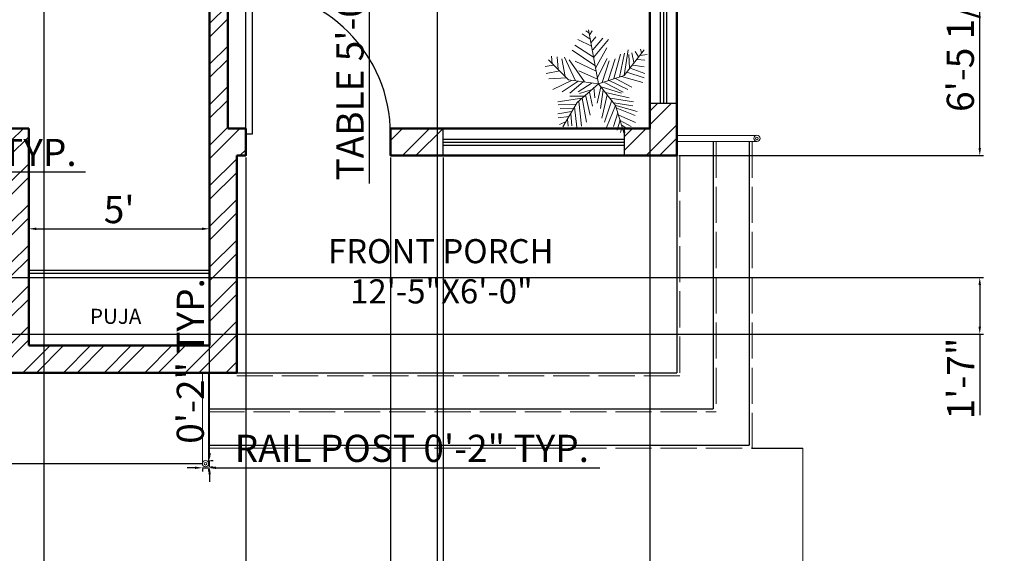
# Model space of a CAD drawing. Units: inches. Extents: x 635 to 1184, y 1837 to 2697.
# Tile 3 of 6: x 857 to 1184, y 2024 to 2201. Entities that reach past the tile are written whole.
import ezdxf

# ---------------------------------------------------------------- set-up
doc = ezdxf.new("R2010")
doc.units = ezdxf.units.IN
doc.linetypes.add('ACAD_ISO02W100', pattern=[15, 12, -3])
for name, color, linetype, lineweight in [('A-ANNO-DIMS', 2, 'Continuous', 18), ('A-ANNO-SYMB', 7, 'Continuous', 18), ('A-AREA-IDEN', 7, 'Continuous', 25), ('A-CSWK', 8, 'Continuous', 25), ('A-DOOR', 4, 'Continuous', 25), ('A-FLOR-RAIL', 7, 'Continuous', 18), ('A-FLOR-STRS', 7, 'Continuous', 25), ('A-FLOR-STRS-HIDN', 8, 'ACAD_ISO02W100', 13), ('A-GLAZ', 244, 'Continuous', 25), ('A-WALL', 7, 'Continuous', 50), ('A-WALL-PATT', 252, 'Continuous', 13), ('C-ROAD', 8, 'Continuous', 25), ('L-PLNT', 94, 'Continuous', 13)]:
    doc.layers.add(name, color=color, linetype=linetype, lineweight=lineweight)
doc.styles.get("Standard").update_dxf_attribs({"font": 'arial.ttf'})
doc.dimstyles.new('ISO-25', dxfattribs={"dimtxt": 9, "dimasz": 2.5, "dimexe": 1.25, "dimexo": 0.625, "dimtad": 1, "dimlunit": 3, "dimtxsty": 'Standard', "dimcen": 2.5, "dimadec": 0, "dimazin": 0, "dimtfac": 1, "dimtmove": 0, "dimatfit": 3, "dimfxl": 1, "dimarcsym": 0})

# ---------------------------------------------------------------- blocks, each defined once
blk = doc.blocks.new('*U3')
for p, q in [((0, 0), (0, -6)), ((40, 0), (40, -6))]:
    blk.add_line(p, q)
blk.add_lwpolyline([(0, 0), (0, 40), (1.75, 40), (1.75, 0)], close=True)
blk.add_arc((0, 0), 40, 0, 90)
blk = doc.blocks.new('*U15')
for p, q in [((-8.737, 47.138), (-17.069, 52.711)), ((-10.186, 53.64), (-13.084, 55.962)), ((0, 0), (-10.5, 57)), ((-9.099, 51.782), (-6.563, 55.962)), ((-7.288, 39.707), (-21.778, 46.673)), ((-7.65, 43.423), (-2.578, 49.46)), ((-5.839, 35.992), (4.667, 48.067)), ((-5.114, 27.632), (10.463, 46.673)), ((-3.665, 19.273), (-27.574, 35.527)), ((-5.114, 28.097), (-24.676, 40.636)), ((-2.941, 16.486), (8.652, 37.85)), ((16.259, 5.805), (23.142, 31.348)), ((22.055, 7.198), (27.489, 32.277)), ((27, 9), (48, 36)), ((27.127, 9.056), (31.112, 35.992)), ((35.096, 32.741), (37.27, 22.524)), ((38.719, 34.134), (41.979, 28.561)), ((44.153, 36.456), (45.239, 32.741)), ((-31.5, 4.5), (-52.5, 25.5)), ((-48.585, 21.131), (-49.309, 29.026)), ((-43.513, 28.561), (-42.427, 15.558)), ((-38.442, 26.239), (-34.819, 7.663)), ((-35.544, 28.097), (-24.314, 3.947)), ((-14.533, 2.09), (-30.834, 25.31)), ((-24.314, 23.917), (-2.941, 13.7)), ((-1.129, 6.734), (9.014, 26.704)), ((3.942, 1.625), (11.187, 24.381)), ((10.101, 3.483), (17.708, 26.239)), ((31.836, 30.883), (32.561, 16.486)), ((40.53, 25.775), (48.862, 24.846)), ((43.791, 29.954), (51.036, 30.883)), ((-47.498, 19.737), (-55.83, 18.344)), ((-40.615, 13.7), (-55.105, 10.913)), ((-20.691, 13.7), (-1.129, 4.876)), ((29.662, 12.307), (48.137, 6.269)), ((33.285, 16.486), (48.862, 10.913)), ((36.183, 19.737), (48.137, 17.88)), ((-33.37, 6.269), (-52.207, 5.34)), ((-28.299, 3.483), (-47.86, -5.805)), ((-21.416, 3.018), (-38.079, -8.128)), ((0, 0), (-31.5, 4.5)), ((-15.982, 2.09), (-30.11, -9.521)), ((0, 0), (-22.5, -19.5)), ((-6.563, 1.161), (-21.416, -8.128)), ((0, 0), (27, 9)), ((0, 0), (18, -22.5)), ((6.478, 1.625), (26.04, -8.592)), ((11.187, 3.483), (30.749, -5.805)), ((18.07, 5.805), (35.096, -3.483)), ((24.229, 7.663), (46.688, 1.625)), ((-6.563, -5.805), (-19.967, -9.985)), ((-9.461, -8.592), (-6.201, -23.453)), ((-4.752, -3.483), (-3.665, -14.629)), ((2.493, -3.019), (-1.491, -20.202)), ((1.769, -2.555), (24.229, -9.521)), ((5.029, -6.27), (2.131, -25.775)), ((7.565, -9.056), (32.198, -14.629)), ((-17.431, -15.094), (-42.789, -18.809)), ((-22.5, -19.5), (-37.5, -45)), ((-15.257, -12.772), (-30.11, -12.772)), ((-20.691, -18.345), (-17.793, -44.352)), ((-17.069, -15.094), (-12.721, -40.172)), ((-13.446, -11.378), (-8.737, -32.741)), ((9.014, -11.378), (3.58, -35.992)), ((14.085, -16.951), (6.478, -40.172)), ((12.274, -15.094), (36.907, -18.809)), ((16.259, -19.738), (36.183, -22.989)), ((-28.299, -29.026), (-42.789, -31.348)), ((-24.314, -21.596), (-42.427, -22.06)), ((-26.849, -26.24), (-40.253, -25.775)), ((-29.023, -30.884), (-27.936, -43.887)), ((-25.038, -23.918), (-22.865, -45.281)), ((18.07, -22.524), (8.289, -45.745)), ((20.244, -30.419), (15.897, -44.816)), ((18, -22.5), (27, -52.5)), ((18.433, -22.524), (40.53, -29.026)), ((19.157, -25.311), (38.719, -33.206)), ((-30.834, -34.135), (-42.427, -35.528)), ((-34.457, -39.708), (-40.978, -42.494)), ((-32.646, -36.921), (-31.921, -44.352)), ((22.78, -37.85), (19.519, -48.532)), ((21.331, -32.741), (39.081, -40.636)), ((22.78, -38.314), (34.372, -44.816)), ((24.591, -45.745), (23.142, -50.854)), ((24.591, -43.423), (30.749, -47.603)), ((26.764, -49.925), (28.213, -50.854))]:
    blk.add_line(p, q)
blk = doc.blocks.new('*D16')
at = {"layer": 'A-ANNO-DIMS', "color": 0, "lineweight": -2, "transparency": 16777216}
for p, q in [((860.28, 2141.58), (860.28, 2130.63)), ((920.28, 2141.58), (920.28, 2130.63)), ((862.78, 2131.88), (917.78, 2131.88))]:
    blk.add_line(p, q, dxfattribs=at)
at = {"layer": 'A-ANNO-DIMS', "color": 0, "transparency": 16777216}
for points in [[(862.78, 2132.29), (862.78, 2131.46), (860.28, 2131.88)], [(917.78, 2132.29), (917.78, 2131.46), (920.28, 2131.88)]]:
    blk.add_solid(points, dxfattribs=at)
at = {"layer": 'DEFPOINTS', "color": 0, "transparency": 16777216}
for p in [(860.28, 2142.2), (920.28, 2142.2), (920.28, 2131.88)]:
    blk.add_point(p, dxfattribs=at)
at = {"layer": 'A-ANNO-DIMS', "color": 0, "transparency": 16777216, "insert": (890.28, 2137.08), "char_height": 9, "attachment_point": 5}
blk.add_mtext("5'", dxfattribs=at)
blk = doc.blocks.new('WIN-60IN')
for p, q in [((0, 5.5), (60, 5.5)), ((0, 4.5), (60, 4.5)), ((0, 3.5), (60, 3.5))]:
    blk.add_line(p, q)
blk.add_lwpolyline([(0, 9), (60, 9), (60, 0), (0, 0)], close=True)
blk = doc.blocks.new('PORCH-RAIL-POST')
for radius in [1.04, 0.436]:
    blk.add_circle((1.04, 1.04), radius)
blk = doc.blocks.new('*D31')
at = {"layer": 'A-ANNO-DIMS', "color": 0, "lineweight": -2, "transparency": 16777216}
for p, q in [((730.76, 2149.5), (730.76, 2152.01)), ((733.26, 2150.76), (740.79, 2150.76)), ((743.29, 2149.5), (743.29, 2152.01)), ((743.29, 2150.76), (879.06, 2150.76))]:
    blk.add_line(p, q, dxfattribs=at)
at = {"layer": 'A-ANNO-DIMS', "color": 0, "transparency": 16777216}
for points in [[(733.26, 2151.18), (733.26, 2150.34), (730.76, 2150.76)], [(740.79, 2151.18), (740.79, 2150.34), (743.29, 2150.76)]]:
    blk.add_solid(points, dxfattribs=at)
at = {"layer": 'DEFPOINTS', "color": 0, "transparency": 16777216}
for p in [(743.29, 2150.76), (730.76, 2148.88), (743.29, 2148.88)]:
    blk.add_point(p, dxfattribs=at)
at = {"layer": 'A-ANNO-DIMS', "color": 0, "transparency": 16777216, "insert": (812.43, 2156.04), "char_height": 9, "attachment_point": 5}
blk.add_mtext('BURNER 1\'-0 1/2" TYP.', dxfattribs=at)
blk = doc.blocks.new('*D33')
at = {"layer": 'A-ANNO-DIMS', "color": 0, "lineweight": -2, "transparency": 16777216}
for p, q in [((915.38, 2052.61), (912.88, 2052.61)), ((917.88, 2052.61), (919.95, 2052.61)), ((917.88, 2052.3), (917.88, 2051.36)), ((919.95, 2052.3), (919.95, 2051.36)), ((922.45, 2052.61), (1049.77, 2052.61))]:
    blk.add_line(p, q, dxfattribs=at)
at = {"layer": 'A-ANNO-DIMS', "color": 0, "transparency": 16777216}
for points in [[(915.38, 2053.03), (915.38, 2052.2), (917.88, 2052.61)], [(922.45, 2053.03), (922.45, 2052.2), (919.95, 2052.61)]]:
    blk.add_solid(points, dxfattribs=at)
at = {"layer": 'DEFPOINTS', "color": 0, "transparency": 16777216}
for p in [(917.88, 2052.93), (919.95, 2052.93), (919.95, 2052.61)]:
    blk.add_point(p, dxfattribs=at)
at = {"layer": 'A-ANNO-DIMS', "color": 0, "transparency": 16777216, "insert": (987.36, 2057.9), "char_height": 9, "attachment_point": 5}
blk.add_mtext('RAIL POST 0\'-2" TYP.', dxfattribs=at)
blk = doc.blocks.new('*D34')
at = {"layer": 'A-ANNO-DIMS', "color": 0, "lineweight": -2, "transparency": 16777216}
for p, q in [((920.26, 2057.5), (920.26, 2116.11)), ((920.26, 2052.93), (920.26, 2055)), ((920.58, 2055), (921.51, 2055)), ((920.58, 2052.93), (921.51, 2052.93)), ((920.26, 2050.43), (920.26, 2047.93))]:
    blk.add_line(p, q, dxfattribs=at)
at = {"layer": 'A-ANNO-DIMS', "color": 0, "transparency": 16777216}
for points in [[(919.85, 2057.5), (920.68, 2057.5), (920.26, 2055)], [(919.85, 2050.43), (920.68, 2050.43), (920.26, 2052.93)]]:
    blk.add_solid(points, dxfattribs=at)
at = {"layer": 'DEFPOINTS', "color": 0, "transparency": 16777216}
for p in [(919.95, 2055), (920.26, 2055), (919.95, 2052.93)]:
    blk.add_point(p, dxfattribs=at)
at = {"layer": 'A-ANNO-DIMS', "color": 0, "transparency": 16777216, "insert": (915.04, 2088.05), "char_height": 9, "attachment_point": 5, "rotation": 90}
blk.add_mtext('0\'-2" TYP.', dxfattribs=at)
blk = doc.blocks.new('*D39')
at = {"layer": 'A-ANNO-DIMS', "color": 0, "lineweight": -2, "transparency": 16777216}
for p, q in [((981.62, 2278.1), (972, 2278.1)), ((973.25, 2275.6), (973.25, 2220.6)), ((981.62, 2218.1), (972, 2218.1)), ((973.25, 2218.1), (973.25, 2146.87))]:
    blk.add_line(p, q, dxfattribs=at)
at = {"layer": 'A-ANNO-DIMS', "color": 0, "transparency": 16777216}
for points in [[(972.83, 2275.6), (973.67, 2275.6), (973.25, 2278.1)], [(972.83, 2220.6), (973.67, 2220.6), (973.25, 2218.1)]]:
    blk.add_solid(points, dxfattribs=at)
at = {"layer": 'DEFPOINTS', "color": 0, "transparency": 16777216}
for p in [(982.25, 2278.1), (973.25, 2218.1), (982.25, 2218.1)]:
    blk.add_point(p, dxfattribs=at)
at = {"layer": 'A-ANNO-DIMS', "color": 0, "transparency": 16777216, "insert": (968.03, 2181.23), "char_height": 9, "attachment_point": 5, "rotation": 90}
blk.add_mtext('TABLE 5\'-0"', dxfattribs=at)
blk = doc.blocks.new('*D49')
at = {"layer": 'A-ANNO-DIMS', "color": 0, "lineweight": -2, "transparency": 16777216}
for p, q in [((932.28, 2155.52), (932.28, 1843.99)), ((980.28, 2155.52), (980.28, 1843.99)), ((934.78, 1845.24), (977.78, 1845.24))]:
    blk.add_line(p, q, dxfattribs=at)
at = {"layer": 'A-ANNO-DIMS', "color": 0, "transparency": 16777216}
for points in [[(934.78, 1845.65), (934.78, 1844.82), (932.28, 1845.24)], [(977.78, 1845.65), (977.78, 1844.82), (980.28, 1845.24)]]:
    blk.add_solid(points, dxfattribs=at)
at = {"layer": 'DEFPOINTS', "color": 0, "transparency": 16777216}
for p in [(932.28, 2156.14), (980.28, 2156.14), (980.28, 1845.24)]:
    blk.add_point(p, dxfattribs=at)
at = {"layer": 'A-ANNO-DIMS', "color": 0, "transparency": 16777216, "insert": (956.28, 1850.46), "char_height": 9, "attachment_point": 5}
blk.add_mtext('4\'-0"', dxfattribs=at)
blk = doc.blocks.new('*D50')
at = {"layer": 'A-ANNO-DIMS', "color": 0, "lineweight": -2, "transparency": 16777216}
for p, q in [((980.28, 2155.52), (980.28, 1843.99)), ((997.78, 2155.52), (997.78, 1843.99)), ((982.78, 1845.24), (995.28, 1845.24)), ((997.78, 1845.24), (1045.58, 1845.24))]:
    blk.add_line(p, q, dxfattribs=at)
at = {"layer": 'A-ANNO-DIMS', "color": 0, "transparency": 16777216}
for points in [[(982.78, 1845.65), (982.78, 1844.82), (980.28, 1845.24)], [(995.28, 1845.65), (995.28, 1844.82), (997.78, 1845.24)]]:
    blk.add_solid(points, dxfattribs=at)
at = {"layer": 'DEFPOINTS', "color": 0, "transparency": 16777216}
for p in [(980.28, 2156.14), (997.78, 2156.14), (997.78, 1845.24)]:
    blk.add_point(p, dxfattribs=at)
at = {"layer": 'A-ANNO-DIMS', "color": 0, "transparency": 16777216, "insert": (1022.93, 1850.52), "char_height": 9, "attachment_point": 5}
blk.add_mtext('1\'-5 1/2"', dxfattribs=at)
blk = doc.blocks.new('*D52')
at = {"layer": 'A-ANNO-DIMS', "color": 0, "lineweight": -2, "transparency": 16777216}
for p, q in [((1075.91, 2233.44), (1176.99, 2233.44)), ((1175.74, 2158.64), (1175.74, 2230.94)), ((1075.91, 2156.14), (1176.99, 2156.14))]:
    blk.add_line(p, q, dxfattribs=at)
at = {"layer": 'A-ANNO-DIMS', "color": 0, "transparency": 16777216}
for points in [[(1175.32, 2230.94), (1176.15, 2230.94), (1175.74, 2233.44)], [(1175.32, 2158.64), (1176.15, 2158.64), (1175.74, 2156.14)]]:
    blk.add_solid(points, dxfattribs=at)
at = {"layer": 'DEFPOINTS', "color": 0, "transparency": 16777216}
for p in [(1075.28, 2233.44), (1175.74, 2233.44), (1075.28, 2156.14)]:
    blk.add_point(p, dxfattribs=at)
at = {"layer": 'A-ANNO-DIMS', "color": 0, "transparency": 16777216, "insert": (1170.46, 2194.79), "char_height": 9, "attachment_point": 5, "rotation": 90}
blk.add_mtext('6\'-5 1/2"', dxfattribs=at)
blk = doc.blocks.new('*D57')
at = {"layer": 'A-ANNO-DIMS', "color": 0, "lineweight": -2, "transparency": 16777216}
for p, q in [((811.77, 2115.72), (1176.99, 2115.72)), ((1175.74, 2113.22), (1175.74, 2099.39)), ((811.77, 2096.89), (1176.99, 2096.89)), ((1175.74, 2096.89), (1175.74, 2070.06))]:
    blk.add_line(p, q, dxfattribs=at)
at = {"layer": 'A-ANNO-DIMS', "color": 0, "transparency": 16777216}
for points in [[(1175.32, 2113.22), (1176.15, 2113.22), (1175.74, 2115.72)], [(1175.32, 2099.39), (1176.15, 2099.39), (1175.74, 2096.89)]]:
    blk.add_solid(points, dxfattribs=at)
at = {"layer": 'DEFPOINTS', "color": 0, "transparency": 16777216}
for p in [(811.15, 2115.72), (811.15, 2096.89), (1175.74, 2096.89)]:
    blk.add_point(p, dxfattribs=at)
at = {"layer": 'A-ANNO-DIMS', "color": 0, "transparency": 16777216, "insert": (1170.59, 2082.22), "char_height": 9, "attachment_point": 5, "rotation": 90}
blk.add_mtext('1\'-7"', dxfattribs=at)
blk = doc.blocks.new('*D62')
at = {"layer": 'A-ANNO-DIMS', "color": 0, "lineweight": -2, "transparency": 16777216}
for p, q in [((829.28, 2442.52), (829.28, 1843.99)), ((865.28, 2442.52), (865.28, 1843.99)), ((831.78, 1845.24), (862.78, 1845.24))]:
    blk.add_line(p, q, dxfattribs=at)
at = {"layer": 'A-ANNO-DIMS', "color": 0, "transparency": 16777216}
for points in [[(831.78, 1845.65), (831.78, 1844.82), (829.28, 1845.24)], [(862.78, 1845.65), (862.78, 1844.82), (865.28, 1845.24)]]:
    blk.add_solid(points, dxfattribs=at)
at = {"layer": 'DEFPOINTS', "color": 0, "transparency": 16777216}
for p in [(829.28, 2443.14), (865.28, 2443.14), (865.28, 1845.24)]:
    blk.add_point(p, dxfattribs=at)
at = {"layer": 'A-ANNO-DIMS', "color": 0, "transparency": 16777216, "insert": (847.28, 1850.46), "char_height": 9, "attachment_point": 5}
blk.add_mtext('3\'-0"', dxfattribs=at)
blk = doc.blocks.new('*D63')
at = {"layer": 'A-ANNO-DIMS', "color": 0, "lineweight": -2, "transparency": 16777216}
for p, q in [((995.78, 2448.52), (995.78, 1843.99)), ((1066.28, 2448.52), (1066.28, 1843.99)), ((998.28, 1845.24), (1063.78, 1845.24))]:
    blk.add_line(p, q, dxfattribs=at)
at = {"layer": 'A-ANNO-DIMS', "color": 0, "transparency": 16777216}
for points in [[(998.28, 1845.65), (998.28, 1844.82), (995.78, 1845.24)], [(1063.78, 1845.65), (1063.78, 1844.82), (1066.28, 1845.24)]]:
    blk.add_solid(points, dxfattribs=at)
at = {"layer": 'DEFPOINTS', "color": 0, "transparency": 16777216}
for p in [(995.78, 2449.14), (1066.28, 2449.14), (1066.28, 1845.24)]:
    blk.add_point(p, dxfattribs=at)
at = {"layer": 'A-ANNO-DIMS', "color": 0, "transparency": 16777216, "insert": (1031.03, 1850.52), "char_height": 9, "attachment_point": 5}
blk.add_mtext('5\'-10 1/2"', dxfattribs=at)

msp = doc.modelspace()

# ---------------------------------------------------------------- hatches: boundary and pattern name
at = {"layer": 'A-WALL-PATT'}
h = msp.add_hatch(dxfattribs=at)
h.set_pattern_fill('ANSI32', color=256)
h.paths.add_polyline_path([(723.282, 2313.142), (714.282, 2313.142), (714.282, 2234.142), (718.782, 2234.142), (723.282, 2234.142), (723.282, 2237.142), (779.782, 2237.142), (779.782, 2243.142), (723.282, 2243.142)])
h.paths.add_polyline_path([(926.282, 2320.142), (920.282, 2320.142), (920.282, 2243.142), (845.782, 2243.142), (845.782, 2237.142), (920.282, 2237.142), (920.282, 2093.142), (860.282, 2093.142), (860.282, 2165.142), (854.282, 2165.142), (854.282, 2093.142), (818.782, 2093.142), (818.782, 2084.142), (929.282, 2084.142), (929.282, 2156.142), (932.282, 2156.142), (932.282, 2165.142), (926.282, 2165.142)])
h.paths.add_polyline_path([(1075.282, 2250.443), (1066.282, 2250.443), (1066.282, 2233.442), (1075.282, 2233.442)])
h.paths.add_polyline_path([(1075.282, 2173.442), (1066.282, 2173.442), (1066.282, 2165.142), (1057.782, 2165.142), (1057.782, 2156.142), (1075.282, 2156.142)])
h.paths.add_polyline_path([(997.782, 2165.142), (980.282, 2165.142), (980.282, 2156.142), (997.782, 2156.142)])
h.paths.add_polyline_path([(1075.282, 2338.142), (1066.282, 2338.142), (1066.282, 2310.443), (1075.282, 2310.443)])
h.paths.add_polyline_path([(758.782, 2093.142), (723.282, 2093.142), (723.282, 2154.642), (714.282, 2154.642), (714.282, 2084.142), (758.782, 2084.142)])
h.paths.add_polyline_path([(723.282, 2204.142), (714.282, 2204.142), (714.282, 2175.642), (723.282, 2175.642)])
h.paths.add_polyline_path([(1075.282, 2404.069), (1066.282, 2404.069), (1066.282, 2383.142), (970.282, 2383.142), (970.282, 2386.142), (964.282, 2386.142), (964.282, 2383.142), (926.282, 2383.142), (926.282, 2389.142), (920.282, 2389.142), (920.282, 2368.142), (926.282, 2368.142), (926.282, 2377.142), (1066.282, 2377.142), (1066.282, 2374.142), (1075.282, 2374.142)])
h.paths.add_polyline_path([(926.282, 2443.142), (964.282, 2443.142), (964.282, 2416.142), (970.282, 2416.142), (970.282, 2443.142), (1066.282, 2443.142), (1066.282, 2425.069), (1075.282, 2425.069), (1075.282, 2503.642), (1066.282, 2503.642), (1066.282, 2449.142), (865.282, 2449.142), (865.282, 2443.142), (920.282, 2443.142), (920.282, 2416.142), (926.282, 2416.142)])
h.paths.add_polyline_path([(829.282, 2449.142), (826.282, 2449.142), (826.282, 2527.142), (826.282, 2557.642), (820.282, 2557.642), (820.282, 2527.142), (817.282, 2527.142), (817.282, 2521.142), (820.282, 2521.142), (820.282, 2449.142), (723.282, 2449.142), (723.282, 2474.642), (714.282, 2474.642), (714.282, 2373.142), (723.282, 2373.142), (723.282, 2443.142), (829.282, 2443.142)])
h.paths.add_polyline_path([(787.282, 2527.142), (723.282, 2527.142), (723.282, 2618.142), (820.282, 2618.142), (820.282, 2587.642), (826.282, 2587.642), (826.282, 2618.142), (916.282, 2618.142), (916.282, 2627.142), (714.282, 2627.142), (714.282, 2495.642), (723.282, 2495.642), (723.282, 2521.142), (787.282, 2521.142)])
h.paths.add_polyline_path([(1075.282, 2627.142), (976.282, 2627.142), (976.282, 2618.142), (1066.282, 2618.142), (1066.282, 2563.642), (1075.282, 2563.642)])

# ---------------------------------------------------------------- linework, layer by layer
at = {"layer": 'A-ANNO-SYMB'}
msp.add_lwpolyline([(1117.034, 2059.142), (1117.034, 2013.802), (1096.782, 2004.337), (1135.238, 2004.087), (1117.034, 1989.817), (1117.034, 1951.962)], dxfattribs=at)
at = {"layer": 'A-CSWK'}
for p, q in [((860.282, 2118.142), (920.282, 2118.142)), ((860.282, 2117.142), (920.282, 2117.142))]:
    msp.add_line(p, q, dxfattribs=at)
at = {"layer": 'A-FLOR-RAIL'}
for p, q in [((1075.282, 2162.817), (1101.428, 2162.817)), ((1075.282, 2160.817), (1101.809, 2160.817)), ((917.88, 2084.142), (917.88, 2053.968)), ((919.88, 2084.142), (919.88, 2054.343))]:
    msp.add_line(p, q, dxfattribs=at)
at = {"layer": 'A-FLOR-STRS'}
for p, q in [((1087.282, 2160.817), (1087.282, 2072.142)), ((1099.282, 2160.817), (1099.282, 2060.142)), ((1075.282, 2156.142), (1075.282, 2084.142)), ((929.282, 2084.142), (1075.282, 2084.142)), ((919.88, 2072.142), (1087.282, 2072.142)), ((919.88, 2060.142), (1099.282, 2060.142))]:
    msp.add_line(p, q, dxfattribs=at)
at = {"layer": 'A-FLOR-STRS-HIDN'}
for p, q in [((1088.282, 2160.817), (1088.282, 2071.142)), ((1100.282, 2160.817), (1100.282, 2059.142)), ((1076.282, 2156.142), (1076.282, 2083.142)), ((929.282, 2083.142), (1076.282, 2083.142)), ((919.88, 2071.142), (1088.282, 2071.142)), ((919.88, 2059.142), (1100.282, 2059.142))]:
    msp.add_line(p, q, dxfattribs=at)
at = {"layer": 'A-WALL'}
for p, q in [((1066.282, 2338.142), (1066.282, 2165.142)), ((1075.282, 2338.142), (1075.282, 2156.142)), ((926.282, 2320.142), (926.282, 2165.142)), ((920.282, 2237.142), (920.282, 2093.142)), ((860.282, 2165.142), (854.282, 2165.142)), ((860.282, 2165.142), (860.282, 2093.142)), ((926.282, 2165.142), (932.282, 2165.142)), ((932.282, 2156.142), (932.282, 2165.142)), ((980.282, 2156.142), (980.282, 2165.142)), ((980.282, 2165.142), (1066.282, 2165.142)), ((929.282, 2156.142), (929.282, 2084.142)), ((929.282, 2156.142), (932.282, 2156.142)), ((980.282, 2156.142), (1075.282, 2156.142)), ((860.282, 2093.142), (920.282, 2093.142)), ((714.282, 2084.142), (929.282, 2084.142))]:
    msp.add_line(p, q, dxfattribs=at)
at = {"layer": 'C-ROAD'}
for p, q in [((1100.282, 2059.142), (1117.034, 2059.142)), ((917.88, 2053.962), (714.282, 2053.962))]:
    msp.add_line(p, q, dxfattribs=at)

# ---------------------------------------------------------------- block references
at = {"layer": 'A-DOOR', "xscale": 1.199999999999993, "yscale": 1.199999999999993, "zscale": 1.199999999999993}
msp.add_blockref('*U3', (932.282, 2163.225), dxfattribs=at)
at = {"layer": 'A-FLOR-RAIL'}
for p in [(1100.773, 2160.817), (917.88, 2052.926)]:
    msp.add_blockref('PORCH-RAIL-POST', p, dxfattribs=at)
at = {"layer": 'A-GLAZ', "rotation": 270.0000000000012}
msp.add_blockref('WIN-60IN', (1066.282, 2233.442), dxfattribs=at)
at = {"layer": 'A-GLAZ'}
msp.add_blockref('WIN-60IN', (997.782, 2156.142), dxfattribs=at)
at = {"layer": 'L-PLNT', "xscale": 0.3157050638920436, "yscale": 0.3157050638920436, "zscale": 0.3157050638920436}
msp.add_blockref('*U15', (1049.256, 2179.912), dxfattribs=at)

# ---------------------------------------------------------------- texts
at = {"layer": 'A-AREA-IDEN', "attachment_point": 1}
for s, width, insert, char_height in [('FRONT PORCH\\P   12\'-5"X6\'-0"', 82.16464, (959.565, 2128.459), 8), ('PUJA', 17.67503, (880.605, 2105.355), 5)]:
    msp.add_mtext_dynamic_manual_height_columns(s, width=width, gutter_width=12.5, heights=[0], dxfattribs=dict(at, insert=insert, char_height=char_height))

# ---------------------------------------------------------------- dimensions: what is measured, and where the dimension line sits
at = {"layer": 'A-ANNO-DIMS'}
for base, p1, p2, override, picture, middle in [((1066.282, 1845.237), (995.782, 2449.142), (1066.282, 2449.142), {"dimdec": 1, "dimlfac": 1, "dimrnd": 0, "dimzin": 1, "dimdsep": 46, "dimlunit": 4, "dimfrac": 2}, '*D63', (1031.032, 1850.516)), ((865.282, 1845.237), (829.282, 2443.142), (865.282, 2443.142), {"dimdec": 1, "dimlfac": 1, "dimrnd": 0, "dimzin": 1, "dimdsep": 46, "dimlunit": 4, "dimfrac": 2}, '*D62', (847.282, 1850.461)), ((980.282, 1845.237), (932.282, 2156.142), (980.282, 2156.142), {"dimdec": 1, "dimlfac": 1, "dimrnd": 0, "dimzin": 1, "dimdsep": 46, "dimlunit": 4, "dimfrac": 2}, '*D49', (956.282, 1850.458)), ((997.782, 1845.237), (980.282, 2156.142), (997.782, 2156.142), {"dimdec": 1, "dimlfac": 1, "dimrnd": 0, "dimzin": 1, "dimdsep": 46, "dimlunit": 4, "dimfrac": 2}, '*D50', (1022.931, 1850.516)), ((920.282, 2131.877), (860.282, 2142.203), (920.282, 2142.203), {"dimclrd": 0, "dimclre": 0, "dimclrt": 0}, '*D16', (890.282, 2137.078))]:
    dim = msp.add_linear_dim(base=base, p1=p1, p2=p2, dimstyle='ISO-25', override=override, dxfattribs=at)
    dim.commit()
    dim.dimension.update_dxf_attribs({"geometry": picture, "text_midpoint": middle})
for base, p1, p2, angle, text, picture, middle in [((973.249, 2218.095), (982.249, 2278.095), (982.249, 2218.095), 270, 'TABLE <>', '*D39', (968.028, 2181.233)), ((920.264, 2054.998), (919.953, 2052.926), (919.953, 2054.998), 90, '<> TYP.', '*D34', (915.043, 2088.053))]:
    dim = msp.add_linear_dim(base=base, p1=p1, p2=p2, angle=angle, text=text, dimstyle='ISO-25', override={"dimdec": 1, "dimlfac": 1, "dimrnd": 0, "dimzin": 1, "dimdsep": 46, "dimlunit": 4, "dimfrac": 2}, dxfattribs=at)
    dim.commit()
    dim.dimension.update_dxf_attribs({"geometry": picture, "text_midpoint": middle})
for base, p1, p2, picture, middle in [((1175.738, 2233.442), (1075.282, 2156.142), (1075.282, 2233.442), '*D52', (1170.459, 2194.792)), ((1175.738, 2096.885), (811.15, 2115.719), (811.15, 2096.885), '*D57', (1170.594, 2082.222))]:
    dim = msp.add_linear_dim(base=base, p1=p1, p2=p2, angle=90, dimstyle='ISO-25', override={"dimdec": 1, "dimlfac": 1, "dimrnd": 0, "dimzin": 1, "dimdsep": 46, "dimlunit": 4, "dimfrac": 2}, dxfattribs=at)
    dim.commit()
    dim.dimension.update_dxf_attribs({"geometry": picture, "text_midpoint": middle})
for base, p1, p2, text, picture, middle in [((743.294, 2150.759), (730.76, 2148.879), (743.294, 2148.879), 'BURNER <> TYP.', '*D31', (812.427, 2156.037)), ((919.953, 2052.615), (917.88, 2052.926), (919.953, 2052.926), 'RAIL POST <> TYP.', '*D33', (987.359, 2057.896))]:
    dim = msp.add_linear_dim(base=base, p1=p1, p2=p2, text=text, dimstyle='ISO-25', override={"dimdec": 1, "dimlfac": 1, "dimrnd": 0, "dimzin": 1, "dimdsep": 46, "dimlunit": 4, "dimfrac": 2}, dxfattribs=at)
    dim.commit()
    dim.dimension.update_dxf_attribs({"geometry": picture, "text_midpoint": middle})

doc.saveas('drawing.dxf')
